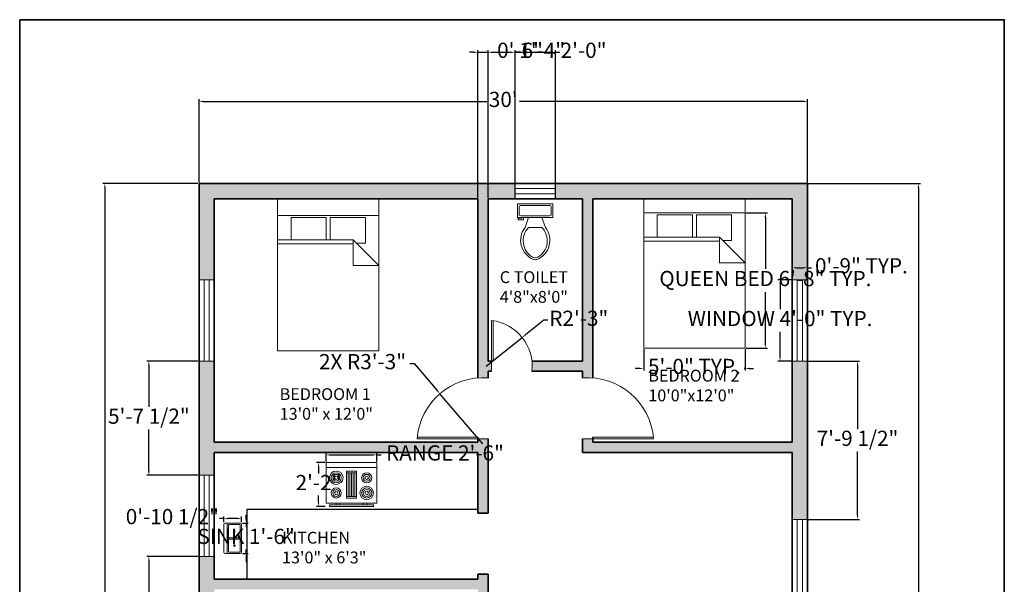
# Model space of a CAD drawing. Units: inches. Extents: x 1994 to 2577, y 1461 to 2158.
# Tile 2 of 2: x 1994 to 2577, y 1824 to 2158. Entities that reach past the tile are written whole.
import ezdxf

# ---------------------------------------------------------------- set-up
doc = ezdxf.new("R2010")
doc.units = ezdxf.units.IN
for name, color, linetype, lineweight in [('A-ANNO-DIMS', 2, 'Continuous', 18), ('A-ANNO-TTLB', 7, 'Continuous', 35), ('A-AREA-IDEN', 7, 'Continuous', 18), ('A-DOOR', 3, 'Continuous', 18), ('A-EQPM', 9, 'Continuous', 18), ('A-FLOR-CASE', 7, 'Continuous', 25), ('A-FLOR-FIXT', 9, 'Continuous', 18), ('A-FURN', 9, 'Continuous', 18), ('A-GLAZ', 4, 'Continuous', 18), ('A-WALL', 7, 'Continuous', 35), ('A-WALL-PATT', 8, 'Continuous', 13)]:
    doc.layers.add(name, color=color, linetype=linetype, lineweight=lineweight)
doc.styles.get("Standard").update_dxf_attribs({"font": 'arial.ttf'})
doc.dimstyles.new('ISO-25', dxfattribs={"dimtxt": 9, "dimasz": 2.5, "dimexe": 1.25, "dimexo": 0.625, "dimgap": 2, "dimtad": 0, "dimtih": 1, "dimtoh": 1, "dimdec": 1, "dimlunit": 4, "dimtxsty": 'Standard', "dimcen": 2.5, "dimadec": 0, "dimazin": 0, "dimtfac": 1, "dimtdec": 1, "dimtmove": 0, "dimatfit": 3, "dimfxl": 1, "dimarcsym": 0})

# ---------------------------------------------------------------- blocks, each defined once
blk = doc.blocks.new('Bed - Queen')
for p, q in [((0, -80.00003), (0, 0)), ((0, 0), (59.99999, 0)), ((59.99999, 0), (59.99999, -80.00003)), ((7.99999, -1.2), (28.79998, -1.2)), ((7.99999, -14.4), (7.99999, -1.2)), ((28.79998, -1.2), (28.79998, -14.4)), ((31.19999, -1.2), (51.99999, -1.2)), ((31.19999, -14.4), (31.19999, -1.2)), ((51.99999, -1.2), (51.99999, -16.4)), ((0, -14.4), (44.8, -14.4)), ((44.8, -16.8), (0, -16.8)), ((59.99999, -29.6), (44.8, -14.4)), ((44.8, -14.4), (44.8, -29.6)), ((51.99999, -16.4), (46.79936, -16.4)), ((44.8, -29.6), (59.99999, -29.6)), ((59.99999, -80.00003), (0, -80.00003))]:
    blk.add_line(p, q)
blk = doc.blocks.new('Sink-double - 36 in top')
for p, q in [((-18, -4), (18, -4)), ((-0.75, -18.5), (-0.75, -6.5)), ((0.75, -6.5), (0.75, -18.5))]:
    blk.add_line(p, q)
for points in [[(-16.5, 0), (16.5, 0)], [(-18, -19.5), (-18, -1.5)], [(-16.5, -18.5), (-16.5, -6.5)], [(-15.5, -5.5), (-1.75, -5.5)], [(1.75, -5.5), (15.5, -5.5)], [(16.5, -6.5), (16.5, -18.5)], [(18, -1.5), (18, -19.5)], [(16.5, -21), (-16.5, -21)], [(-1.75, -19.5), (-15.5, -19.5)], [(15.5, -19.5), (1.75, -19.5)]]:
    blk.add_lwpolyline(points)
for centre, radius in [((-8.5, -12.5), 1), ((8.5, -12.5), 1), ((-8.5, -12.5), 0.5), ((8.5, -12.5), 0.5)]:
    blk.add_circle(centre, radius)
for centre, radius, start, end in [((-16.5, -1.5), 1.5, 90, 180), ((16.5, -1.5), 1.5, 0, 90), ((-15.5, -6.5), 1, 90, 180), ((-1.75, -6.5), 1, 0, 90), ((1.75, -6.5), 1, 90, 180), ((15.5, -6.5), 1, 0, 90), ((-16.5, -19.5), 1.5, 180, 270), ((-15.5, -18.5), 1, 180, 270), ((-1.75, -18.5), 1, 270, 0), ((1.75, -18.5), 1, 180, 270), ((15.5, -18.5), 1, 270, 0), ((16.5, -19.5), 1.5, 270, 0)]:
    blk.add_arc(centre, radius, start, end)
blk = doc.blocks.new('Range-Oven - 30 in top')
for p, q in [((0, -3), (30, -3)), ((12, -6), (18, -6)), ((13, -20), (13, -6)), ((14, -6), (14, -20)), ((15, -20), (15, -6)), ((16, -6), (16, -20)), ((17, -20), (17, -6)), ((18, -20), (12, -20)), ((6, -24), (6, -25)), ((8, -25), (8, -24)), ((22, -25), (22, -24)), ((24, -24), (24, -25))]:
    blk.add_line(p, q)
for points in [[(0, -24), (0, 0), (30, 0), (30, -24)], [(12, -21), (12, -5), (18, -5), (18, -21)], [(2, -26), (2, -25), (28, -25), (28, -26)]]:
    blk.add_lwpolyline(points, close=True)
for centre, radius in [((6, -9), 4), ((6, -9), 3), ((6, -9), 2), ((6, -9), 1), ((24, -9), 3), ((24, -9), 2), ((24, -9), 1), ((6, -18), 3), ((6, -18), 2), ((6, -18), 1), ((24, -18), 4), ((24, -18), 3), ((24, -18), 2), ((24, -18), 1)]:
    blk.add_circle(centre, radius)
blk = doc.blocks.new('*D4')
at = {"layer": 'A-ANNO-DIMS', "color": 0, "lineweight": -2, "transparency": 16777216}
for p, q in [((2461.02, 2061.02), (2527.29, 2061.02)), ((2526.04, 2058.52), (2526.04, 1797.59)), ((2526.04, 1523.52), (2526.04, 1784.44)), ((2461.02, 1521.02), (2527.29, 1521.02))]:
    blk.add_line(p, q, dxfattribs=at)
at = {"layer": 'A-ANNO-DIMS', "color": 0, "transparency": 16777216}
for points in [[(2525.63, 2058.52), (2526.46, 2058.52), (2526.04, 2061.02)], [(2525.63, 1523.52), (2526.46, 1523.52), (2526.04, 1521.02)]]:
    blk.add_solid(points, dxfattribs=at)
at = {"layer": 'Defpoints', "color": 0, "transparency": 16777216}
for p in [(2460.39, 2061.02), (2460.39, 1521.02), (2526.04, 1521.02)]:
    blk.add_point(p, dxfattribs=at)
at = {"layer": 'A-ANNO-DIMS', "color": 0, "transparency": 16777216, "insert": (2526.04, 1791.02), "char_height": 9, "attachment_point": 5}
blk.add_mtext("45'", dxfattribs=at)
blk = doc.blocks.new('*D5')
at = {"layer": 'A-ANNO-DIMS', "color": 0, "lineweight": -2, "transparency": 16777216}
for p, q in [((2100.39, 2061.64), (2100.39, 2110.85)), ((2102.89, 2109.6), (2270.76, 2109.6)), ((2457.89, 2109.6), (2290.02, 2109.6)), ((2460.39, 2061.64), (2460.39, 2110.85))]:
    blk.add_line(p, q, dxfattribs=at)
at = {"layer": 'A-ANNO-DIMS', "color": 0, "transparency": 16777216}
for points in [[(2102.89, 2110.02), (2102.89, 2109.18), (2100.39, 2109.6)], [(2457.89, 2110.02), (2457.89, 2109.18), (2460.39, 2109.6)]]:
    blk.add_solid(points, dxfattribs=at)
at = {"layer": 'Defpoints', "color": 0, "transparency": 16777216}
for p in [(2460.39, 2109.6), (2100.39, 2061.02), (2460.39, 2061.02)]:
    blk.add_point(p, dxfattribs=at)
at = {"layer": 'A-ANNO-DIMS', "color": 0, "transparency": 16777216, "insert": (2280.39, 2109.6), "char_height": 9, "attachment_point": 5}
blk.add_mtext("30'", dxfattribs=at)
blk = doc.blocks.new('*U7')
for p, q in [((9.5, -6), (9.5, -2)), ((-10, -8.5), (-8, -8.5)), ((-10, -9.5), (-10, -8.5)), ((-7, -9.5), (-10, -9.5)), ((-8, -8.5), (-8, -8)), ((-7, -8), (-7, -9.5)), ((-4, -8), (-6, -14)), ((4, -8), (6, -14)), ((4, -14), (-4, -14))]:
    blk.add_line(p, q)
blk.add_lwpolyline([(10.5, -8), (10.5, 0), (-10.5, 0), (-10.5, -8)], close=True)
for points in [[(-9.5, -2), (-9.5, -6)], [(8.5, -1), (-8.5, -1)], [(-8.5, -7), (8.5, -7)]]:
    blk.add_lwpolyline(points)
for centre, radius, start, end in [((-8.62, -1.88), 0.884, 81.8699, 188.1301), ((8.62, -1.88), 0.884, 351.8699, 98.1301), ((-8.62, -6.12), 0.884, 171.8699, 278.1301), ((8.62, -6.12), 0.884, 261.8699, 8.1301), ((3.52, -21.58), 12.17, 141.46911, 247.97143), ((4.2, -21.82), 11.33, 136.36773, 238.94682), ((-3.52, -21.58), 12.17, 292.02843, 38.53071), ((-4.2, -21.82), 11.33, 301.05301, 43.63209), ((0, -27.88), 4, 245.73182, 294.26817), ((0, -29), 4, 254.86053, 285.13947)]:
    blk.add_arc(centre, radius, start, end)
blk = doc.blocks.new('*D8')
at = {"layer": 'A-ANNO-DIMS', "color": 0, "lineweight": -2, "transparency": 16777216}
for p, q in [((2099.77, 2061.02), (2043.44, 2061.02)), ((2044.69, 2058.52), (2044.69, 1797.59)), ((2044.69, 1523.52), (2044.69, 1784.44)), ((2099.77, 1521.02), (2043.44, 1521.02))]:
    blk.add_line(p, q, dxfattribs=at)
at = {"layer": 'A-ANNO-DIMS', "color": 0, "transparency": 16777216}
for points in [[(2044.27, 2058.52), (2045.11, 2058.52), (2044.69, 2061.02)], [(2044.27, 1523.52), (2045.11, 1523.52), (2044.69, 1521.02)]]:
    blk.add_solid(points, dxfattribs=at)
at = {"layer": 'Defpoints', "color": 0, "transparency": 16777216}
for p in [(2100.39, 2061.02), (2044.69, 1521.02), (2100.39, 1521.02)]:
    blk.add_point(p, dxfattribs=at)
at = {"layer": 'A-ANNO-DIMS', "color": 0, "transparency": 16777216, "insert": (2044.69, 1791.02), "char_height": 9, "attachment_point": 5}
blk.add_mtext("45'", dxfattribs=at)
blk = doc.blocks.new('WIN-48IN')
for p, q in [((9, 48), (0, 48)), ((0, 48), (0, 0)), ((3, 48), (3, 0)), ((6, 48), (6, 0)), ((9, 0), (0, 0))]:
    blk.add_line(p, q)
blk = doc.blocks.new('DOOR-SWING-36IN')
for p, q in [((36, 1), (0, 1)), ((36, 0), (0, 0)), ((36, 0), (42, 0))]:
    blk.add_line(p, q)
blk.add_arc((39, -3), 39.12, 85.60129, 175.60129)
blk = doc.blocks.new('*D11')
at = {"layer": 'A-ANNO-DIMS', "color": 0, "lineweight": -2, "transparency": 16777216}
for p, q in [((2450.77, 2004.02), (2442.94, 2004.02)), ((2444.19, 2001.52), (2444.19, 1986.67)), ((2444.19, 1958.52), (2444.19, 1973.36)), ((2450.77, 1956.02), (2442.94, 1956.02))]:
    blk.add_line(p, q, dxfattribs=at)
at = {"layer": 'A-ANNO-DIMS', "color": 0, "transparency": 16777216}
for points in [[(2443.77, 2001.52), (2444.61, 2001.52), (2444.19, 2004.02)], [(2443.77, 1958.52), (2444.61, 1958.52), (2444.19, 1956.02)]]:
    blk.add_solid(points, dxfattribs=at)
at = {"layer": 'Defpoints', "color": 0, "transparency": 16777216}
for p in [(2444.19, 2004.02), (2451.39, 2004.02), (2451.39, 1956.02)]:
    blk.add_point(p, dxfattribs=at)
at = {"layer": 'A-ANNO-DIMS', "color": 0, "transparency": 16777216, "insert": (2444.19, 1980.02), "char_height": 9, "attachment_point": 5}
blk.add_mtext('WINDOW 4\'-0" TYP.', dxfattribs=at)
blk = doc.blocks.new('*D12')
at = {"layer": 'A-ANNO-DIMS', "color": 0, "lineweight": -2, "transparency": 16777216}
for p, q in [((2451.39, 2004.64), (2451.39, 2012.47)), ((2453.89, 2011.22), (2457.89, 2011.22)), ((2460.39, 2004.64), (2460.39, 2012.47)), ((2460.39, 2011.22), (2462.89, 2011.22))]:
    blk.add_line(p, q, dxfattribs=at)
at = {"layer": 'A-ANNO-DIMS', "color": 0, "transparency": 16777216}
for points in [[(2453.89, 2011.63), (2453.89, 2010.8), (2451.39, 2011.22)], [(2457.89, 2011.63), (2457.89, 2010.8), (2460.39, 2011.22)]]:
    blk.add_solid(points, dxfattribs=at)
at = {"layer": 'Defpoints', "color": 0, "transparency": 16777216}
for p in [(2460.39, 2011.22), (2451.39, 2004.02), (2460.39, 2004.02)]:
    blk.add_point(p, dxfattribs=at)
at = {"layer": 'A-ANNO-DIMS', "color": 0, "transparency": 16777216, "insert": (2492.32, 2011.22), "char_height": 9, "attachment_point": 5}
blk.add_mtext('0\'-9" TYP.', dxfattribs=at)
blk = doc.blocks.new('*D15')
at = {"layer": 'A-ANNO-DIMS', "color": 0, "lineweight": -2, "transparency": 16777216}
for p, q in [((2424.13, 2043.69), (2436.75, 2043.69)), ((2435.5, 2041.19), (2435.5, 2010.62)), ((2435.5, 1966.19), (2435.5, 1996.76)), ((2424.13, 1963.69), (2436.75, 1963.69))]:
    blk.add_line(p, q, dxfattribs=at)
at = {"layer": 'A-ANNO-DIMS', "color": 0, "transparency": 16777216}
for points in [[(2435.09, 2041.19), (2435.92, 2041.19), (2435.5, 2043.69)], [(2435.09, 1966.19), (2435.92, 1966.19), (2435.5, 1963.69)]]:
    blk.add_solid(points, dxfattribs=at)
at = {"layer": 'Defpoints', "color": 0, "transparency": 16777216}
for p in [(2423.5, 2043.69), (2435.5, 2043.69), (2423.5, 1963.69)]:
    blk.add_point(p, dxfattribs=at)
at = {"layer": 'A-ANNO-DIMS', "color": 0, "transparency": 16777216, "insert": (2435.5, 2003.69), "char_height": 9, "attachment_point": 5}
blk.add_mtext('QUEEN BED 6\'-8" TYP.', dxfattribs=at)
blk = doc.blocks.new('*D16')
at = {"layer": 'A-ANNO-DIMS', "color": 0, "lineweight": -2, "transparency": 16777216}
for p, q in [((2363.5, 1963.07), (2363.5, 1950.44)), ((2423.5, 1963.07), (2423.5, 1950.44)), ((2361, 1951.69), (2358.5, 1951.69)), ((2363.5, 1951.69), (2364.07, 1951.69)), ((2423.5, 1951.69), (2422.93, 1951.69)), ((2426, 1951.69), (2428.5, 1951.69))]:
    blk.add_line(p, q, dxfattribs=at)
at = {"layer": 'A-ANNO-DIMS', "color": 0, "transparency": 16777216}
for points in [[(2361, 1952.11), (2361, 1951.28), (2363.5, 1951.69)], [(2426, 1952.11), (2426, 1951.28), (2423.5, 1951.69)]]:
    blk.add_solid(points, dxfattribs=at)
at = {"layer": 'Defpoints', "color": 0, "transparency": 16777216}
for p in [(2363.5, 1963.69), (2423.5, 1963.69), (2423.5, 1951.69)]:
    blk.add_point(p, dxfattribs=at)
at = {"layer": 'A-ANNO-DIMS', "color": 0, "transparency": 16777216, "insert": (2393.5, 1951.69), "char_height": 9, "attachment_point": 5}
blk.add_mtext('5\'-0" TYP.', dxfattribs=at)
blk = doc.blocks.new('*D17')
at = {"layer": 'A-ANNO-DIMS', "color": 0, "lineweight": -2, "transparency": 16777216}
for p, q in [((2128.26, 1862.68), (2128.26, 1865.18)), ((2126.19, 1860.18), (2129.51, 1860.18)), ((2128.26, 1860.18), (2128.26, 1857.84)), ((2126.19, 1842.18), (2129.51, 1842.18)), ((2128.26, 1842.18), (2128.26, 1844.53)), ((2128.26, 1839.68), (2128.26, 1837.18))]:
    blk.add_line(p, q, dxfattribs=at)
at = {"layer": 'A-ANNO-DIMS', "color": 0, "transparency": 16777216}
for points in [[(2127.85, 1862.68), (2128.68, 1862.68), (2128.26, 1860.18)], [(2127.85, 1839.68), (2128.68, 1839.68), (2128.26, 1842.18)]]:
    blk.add_solid(points, dxfattribs=at)
at = {"layer": 'Defpoints', "color": 0, "transparency": 16777216}
for p in [(2125.57, 1860.18), (2128.26, 1860.18), (2125.57, 1842.18)]:
    blk.add_point(p, dxfattribs=at)
at = {"layer": 'A-ANNO-DIMS', "color": 0, "transparency": 16777216, "insert": (2128.26, 1851.18), "char_height": 9, "attachment_point": 5}
blk.add_mtext('SINK 1\'-6"', dxfattribs=at)
blk = doc.blocks.new('*D18')
at = {"layer": 'A-ANNO-DIMS', "color": 0, "lineweight": -2, "transparency": 16777216}
for p, q in [((2115.07, 1862.88), (2112.57, 1862.88)), ((2115.07, 1860.81), (2115.07, 1864.13)), ((2123.07, 1862.88), (2117.57, 1862.88)), ((2125.57, 1860.81), (2125.57, 1864.13))]:
    blk.add_line(p, q, dxfattribs=at)
at = {"layer": 'A-ANNO-DIMS', "color": 0, "transparency": 16777216}
for points in [[(2117.57, 1863.3), (2117.57, 1862.46), (2115.07, 1862.88)], [(2123.07, 1863.3), (2123.07, 1862.46), (2125.57, 1862.88)]]:
    blk.add_solid(points, dxfattribs=at)
at = {"layer": 'Defpoints', "color": 0, "transparency": 16777216}
for p in [(2115.07, 1862.88), (2115.07, 1860.18), (2125.57, 1860.18)]:
    blk.add_point(p, dxfattribs=at)
at = {"layer": 'A-ANNO-DIMS', "color": 0, "transparency": 16777216, "insert": (2084.62, 1862.88), "char_height": 9, "attachment_point": 5}
blk.add_mtext('0\'-10 1/2"', dxfattribs=at)
blk = doc.blocks.new('*D19')
at = {"layer": 'A-ANNO-DIMS', "color": 0, "lineweight": -2, "transparency": 16777216}
for p, q in [((2175.6, 1896.64), (2175.6, 1901.77)), ((2178.1, 1900.52), (2203.1, 1900.52)), ((2205.6, 1896.64), (2205.6, 1901.77)), ((2205.6, 1900.52), (2208.1, 1900.52))]:
    blk.add_line(p, q, dxfattribs=at)
at = {"layer": 'A-ANNO-DIMS', "color": 0, "transparency": 16777216}
for points in [[(2178.1, 1900.94), (2178.1, 1900.1), (2175.6, 1900.52)], [(2203.1, 1900.94), (2203.1, 1900.1), (2205.6, 1900.52)]]:
    blk.add_solid(points, dxfattribs=at)
at = {"layer": 'Defpoints', "color": 0, "transparency": 16777216}
for p in [(2205.6, 1900.52), (2175.6, 1896.02), (2205.6, 1896.02)]:
    blk.add_point(p, dxfattribs=at)
at = {"layer": 'A-ANNO-DIMS', "color": 0, "transparency": 16777216, "insert": (2245.93, 1900.52), "char_height": 9, "attachment_point": 5}
blk.add_mtext('RANGE 2\'-6"', dxfattribs=at)
blk = doc.blocks.new('*D20')
at = {"layer": 'A-ANNO-DIMS', "color": 0, "lineweight": -2, "transparency": 16777216}
for p, q in [((2174.98, 1896.02), (2169.85, 1896.02)), ((2171.1, 1893.52), (2171.1, 1889.54)), ((2171.1, 1872.52), (2171.1, 1876.5)), ((2174.98, 1870.02), (2169.85, 1870.02))]:
    blk.add_line(p, q, dxfattribs=at)
at = {"layer": 'A-ANNO-DIMS', "color": 0, "transparency": 16777216}
for points in [[(2170.69, 1893.52), (2171.52, 1893.52), (2171.1, 1896.02)], [(2170.69, 1872.52), (2171.52, 1872.52), (2171.1, 1870.02)]]:
    blk.add_solid(points, dxfattribs=at)
at = {"layer": 'Defpoints', "color": 0, "transparency": 16777216}
for p in [(2171.1, 1896.02), (2175.6, 1896.02), (2175.6, 1870.02)]:
    blk.add_point(p, dxfattribs=at)
at = {"layer": 'A-ANNO-DIMS', "color": 0, "transparency": 16777216, "insert": (2171.1, 1883.02), "char_height": 9, "attachment_point": 5}
blk.add_mtext('2\'-2"', dxfattribs=at)
blk = doc.blocks.new('*D22')
at = {"layer": 'A-ANNO-DIMS', "color": 0, "lineweight": -2, "transparency": 16777216}
for p, q in [((2262.89, 2138.65), (2260.39, 2138.65)), ((2265.39, 2052.64), (2265.39, 2139.9)), ((2265.39, 2138.65), (2271.39, 2138.65)), ((2271.39, 2052.64), (2271.39, 2139.9)), ((2273.89, 2138.65), (2276.39, 2138.65))]:
    blk.add_line(p, q, dxfattribs=at)
at = {"layer": 'A-ANNO-DIMS', "color": 0, "transparency": 16777216}
for points in [[(2262.89, 2139.07), (2262.89, 2138.23), (2265.39, 2138.65)], [(2273.89, 2139.07), (2273.89, 2138.23), (2271.39, 2138.65)]]:
    blk.add_solid(points, dxfattribs=at)
at = {"layer": 'Defpoints', "color": 0, "transparency": 16777216}
for p in [(2271.39, 2138.65), (2265.39, 2052.02), (2271.39, 2052.02)]:
    blk.add_point(p, dxfattribs=at)
at = {"layer": 'A-ANNO-DIMS', "color": 0, "transparency": 16777216, "insert": (2290.35, 2138.65), "char_height": 9, "attachment_point": 5}
blk.add_mtext('0\'-6"', dxfattribs=at)
blk = doc.blocks.new('*D29')
at = {"layer": 'A-ANNO-DIMS', "color": 0, "lineweight": -2, "transparency": 16777216}
for p, q in [((2461.02, 1956.02), (2491.29, 1956.02)), ((2490.04, 1953.52), (2490.04, 1915.83)), ((2490.04, 1864.84), (2490.04, 1902.53)), ((2461.02, 1862.34), (2491.29, 1862.34))]:
    blk.add_line(p, q, dxfattribs=at)
at = {"layer": 'A-ANNO-DIMS', "color": 0, "transparency": 16777216}
for points in [[(2489.62, 1953.52), (2490.46, 1953.52), (2490.04, 1956.02)], [(2489.62, 1864.84), (2490.46, 1864.84), (2490.04, 1862.34)]]:
    blk.add_solid(points, dxfattribs=at)
at = {"layer": 'Defpoints', "color": 0, "transparency": 16777216}
for p in [(2460.39, 1956.02), (2490.04, 1956.02), (2460.39, 1862.34)]:
    blk.add_point(p, dxfattribs=at)
at = {"layer": 'A-ANNO-DIMS', "color": 0, "transparency": 16777216, "insert": (2490.04, 1909.18), "char_height": 9, "attachment_point": 5}
blk.add_mtext('7\'-9 1/2"', dxfattribs=at)
blk = doc.blocks.new('*D31')
at = {"layer": 'A-ANNO-DIMS', "color": 0, "lineweight": -2, "transparency": 16777216}
for p, q in [((2099.77, 1840.52), (2069.49, 1840.52)), ((2070.74, 1838.02), (2070.74, 1816.42)), ((2070.74, 1781.52), (2070.74, 1803.11)), ((2099.77, 1779.02), (2069.49, 1779.02))]:
    blk.add_line(p, q, dxfattribs=at)
at = {"layer": 'A-ANNO-DIMS', "color": 0, "transparency": 16777216}
for points in [[(2070.32, 1838.02), (2071.16, 1838.02), (2070.74, 1840.52)], [(2070.32, 1781.52), (2071.16, 1781.52), (2070.74, 1779.02)]]:
    blk.add_solid(points, dxfattribs=at)
at = {"layer": 'Defpoints', "color": 0, "transparency": 16777216}
for p in [(2070.74, 1840.52), (2100.39, 1840.52), (2100.39, 1779.02)]:
    blk.add_point(p, dxfattribs=at)
at = {"layer": 'A-ANNO-DIMS', "color": 0, "transparency": 16777216, "insert": (2070.74, 1809.77), "char_height": 9, "attachment_point": 5}
blk.add_mtext('5\'-1 1/2"', dxfattribs=at)
blk = doc.blocks.new('*D32')
at = {"layer": 'A-ANNO-DIMS', "color": 0, "lineweight": -2, "transparency": 16777216}
for p, q in [((2099.77, 1956.02), (2069.49, 1956.02)), ((2070.74, 1953.52), (2070.74, 1928.92)), ((2070.74, 1891.02), (2070.74, 1915.61)), ((2099.77, 1888.52), (2069.49, 1888.52))]:
    blk.add_line(p, q, dxfattribs=at)
at = {"layer": 'A-ANNO-DIMS', "color": 0, "transparency": 16777216}
for points in [[(2070.32, 1953.52), (2071.16, 1953.52), (2070.74, 1956.02)], [(2070.32, 1891.02), (2071.16, 1891.02), (2070.74, 1888.52)]]:
    blk.add_solid(points, dxfattribs=at)
at = {"layer": 'Defpoints', "color": 0, "transparency": 16777216}
for p in [(2070.74, 1956.02), (2100.39, 1956.02), (2100.39, 1888.52)]:
    blk.add_point(p, dxfattribs=at)
at = {"layer": 'A-ANNO-DIMS', "color": 0, "transparency": 16777216, "insert": (2070.74, 1922.27), "char_height": 9, "attachment_point": 5}
blk.add_mtext('5\'-7 1/2"', dxfattribs=at)
blk = doc.blocks.new('*D33')
at = {"layer": 'A-ANNO-DIMS', "color": 0, "lineweight": -2, "transparency": 16777216}
for p, q in [((2287.39, 2052.64), (2287.39, 2139.9)), ((2289.89, 2138.65), (2308.89, 2138.65)), ((2311.39, 2052.64), (2311.39, 2139.9)), ((2311.39, 2138.65), (2313.89, 2138.65))]:
    blk.add_line(p, q, dxfattribs=at)
at = {"layer": 'A-ANNO-DIMS', "color": 0, "transparency": 16777216}
for points in [[(2289.89, 2139.07), (2289.89, 2138.23), (2287.39, 2138.65)], [(2308.89, 2139.07), (2308.89, 2138.23), (2311.39, 2138.65)]]:
    blk.add_solid(points, dxfattribs=at)
at = {"layer": 'Defpoints', "color": 0, "transparency": 16777216}
for p in [(2311.39, 2138.65), (2287.39, 2052.02), (2311.39, 2052.02)]:
    blk.add_point(p, dxfattribs=at)
at = {"layer": 'A-ANNO-DIMS', "color": 0, "transparency": 16777216, "insert": (2327.93, 2138.65), "char_height": 9, "attachment_point": 5}
blk.add_mtext('2\'-0"', dxfattribs=at)
blk = doc.blocks.new('*D34')
at = {"layer": 'A-ANNO-DIMS', "color": 0, "lineweight": -2, "transparency": 16777216}
for p, q in [((2271.39, 2052.64), (2271.39, 2139.9)), ((2273.89, 2138.65), (2284.89, 2138.65)), ((2287.39, 2052.64), (2287.39, 2139.9)), ((2287.39, 2138.65), (2289.89, 2138.65))]:
    blk.add_line(p, q, dxfattribs=at)
at = {"layer": 'A-ANNO-DIMS', "color": 0, "transparency": 16777216}
for points in [[(2273.89, 2139.07), (2273.89, 2138.23), (2271.39, 2138.65)], [(2284.89, 2139.07), (2284.89, 2138.23), (2287.39, 2138.65)]]:
    blk.add_solid(points, dxfattribs=at)
at = {"layer": 'Defpoints', "color": 0, "transparency": 16777216}
for p in [(2287.39, 2138.65), (2271.39, 2052.02), (2287.39, 2052.02)]:
    blk.add_point(p, dxfattribs=at)
at = {"layer": 'A-ANNO-DIMS', "color": 0, "transparency": 16777216, "insert": (2303.43, 2138.65), "char_height": 9, "attachment_point": 5}
blk.add_mtext('1\'-4"', dxfattribs=at)
blk = doc.blocks.new('*D40')
at = {"layer": 'A-ANNO-DIMS', "color": 0, "lineweight": -2, "transparency": 16777216}
for p, q in [((2225.16, 1954.53), (2227.66, 1954.53)), ((2227.66, 1954.53), (2241.31, 1938.61)), ((2268.39, 1907.02), (2242.93, 1936.71))]:
    blk.add_line(p, q, dxfattribs=at)
at = {"layer": 'A-ANNO-DIMS', "color": 0, "transparency": 16777216}
blk.add_solid([(2241.62, 1938.88), (2240.99, 1938.34), (2242.93, 1936.71)], dxfattribs=at)
at = {"layer": 'Defpoints', "color": 0, "transparency": 16777216}
for p in [(2242.93, 1936.71), (2268.39, 1907.02)]:
    blk.add_point(p, dxfattribs=at)
at = {"layer": 'A-ANNO-DIMS', "color": 0, "transparency": 16777216, "insert": (2197.15, 1954.53), "char_height": 9, "attachment_point": 5}
blk.add_mtext('2X R3\'-3"', dxfattribs=at)
blk = doc.blocks.new('*D41')
at = {"layer": 'A-ANNO-DIMS', "color": 0, "lineweight": -2, "transparency": 16777216}
for p, q in [((2304.33, 1980.17), (2293.56, 1971.55)), ((2306.83, 1980.17), (2304.33, 1980.17)), ((2270.39, 1953.02), (2291.6, 1969.99))]:
    blk.add_line(p, q, dxfattribs=at)
at = {"layer": 'A-ANNO-DIMS', "color": 0, "transparency": 16777216}
blk.add_solid([(2293.3, 1971.87), (2293.82, 1971.22), (2291.6, 1969.99)], dxfattribs=at)
at = {"layer": 'Defpoints', "color": 0, "transparency": 16777216}
for p in [(2291.6, 1969.99), (2270.39, 1953.02)]:
    blk.add_point(p, dxfattribs=at)
at = {"layer": 'A-ANNO-DIMS', "color": 0, "transparency": 16777216, "insert": (2325.1, 1980.17), "char_height": 9, "attachment_point": 5}
blk.add_mtext('R2\'-3"', dxfattribs=at)

msp = doc.modelspace()

# ---------------------------------------------------------------- hatches: boundary and pattern name
at = {"layer": 'A-WALL-PATT'}
h = msp.add_hatch(color=256, dxfattribs=at)
h.dxf.hatch_style = 1
h.paths.add_polyline_path([(2287.39, 2061.02), (2100.39, 2061.02), (2100.39, 2004.02), (2109.39, 2004.02), (2109.39, 2052.02), (2265.39, 2052.02), (2265.39, 1946.02, -0.038405), (2271.39, 1946.02), (2271.39, 1950.02), (2273.39, 1950.02), (2273.39, 1956.02), (2271.39, 1956.02), (2271.39, 2052.02), (2287.39, 2052.02)])
h.paths.add_polyline_path([(2460.39, 2061.02), (2311.39, 2061.02), (2311.39, 2052.02), (2327.39, 2052.02), (2327.39, 1956.02), (2297.39, 1956.02, -0.055385), (2297.39, 1950.02), (2327.39, 1950.02), (2327.39, 1946.02, -0.038405), (2333.39, 1946.02), (2333.39, 2052.02), (2451.39, 2052.02), (2451.39, 2004.02), (2460.39, 2004.02)])
h.paths.add_polyline_path([(2460.39, 1956.02), (2451.39, 1956.02), (2451.39, 1908.02), (2333.39, 1908.02), (2333.39, 1910.02), (2327.39, 1910.02), (2327.39, 1902.02), (2451.39, 1902.02), (2451.39, 1862.34), (2460.39, 1862.34)])
h.paths.add_polyline_path([(2109.39, 1956.02), (2100.39, 1956.02), (2100.39, 1888.52), (2109.39, 1888.52), (2109.39, 1902.02), (2265.39, 1902.02), (2265.39, 1866.02), (2271.39, 1866.02), (2271.39, 1910.02), (2265.39, 1910.02), (2265.39, 1908.02), (2109.39, 1908.02)])
h.paths.add_polyline_path([(2460.39, 1814.34), (2451.39, 1814.34), (2451.39, 1686.53), (2460.39, 1686.53)])
h.paths.add_polyline_path([(2271.39, 1830.02), (2265.39, 1830.02), (2265.39, 1827.02), (2109.39, 1827.02), (2109.39, 1840.52), (2100.39, 1840.52), (2100.39, 1779.02), (2109.39, 1779.02), (2109.39, 1821.02), (2265.39, 1821.02), (2265.39, 1729.02, -0.038405), (2271.39, 1729.02)])
h.paths.add_polyline_path([(2109.39, 1683.02), (2265.39, 1683.02), (2265.39, 1679.02), (2271.39, 1679.02), (2271.39, 1693.02), (2265.39, 1693.02), (2265.39, 1689.02), (2109.39, 1689.02), (2109.39, 1731.02), (2100.39, 1731.02), (2100.39, 1521.02), (2163.39, 1521.02), (2163.39, 1530.02), (2109.39, 1530.02)])
h.paths.add_polyline_path([(2273.39, 1530.02), (2271.39, 1530.02), (2271.39, 1606.02), (2273.39, 1606.02, -0.038405), (2273.39, 1612.02), (2271.39, 1612.02), (2271.39, 1643.02, -0.038405), (2265.39, 1643.02), (2265.39, 1530.02), (2211.39, 1530.02), (2211.39, 1521.02), (2273.39, 1521.02)])
h.paths.add_polyline_path([(2460.39, 1544.02), (2451.39, 1544.02), (2451.39, 1530.02), (2309.39, 1530.02, -0.055385), (2309.39, 1521.02), (2460.39, 1521.02)])
h.paths.add_polyline_path([(2460.39, 1638.53), (2451.39, 1638.53), (2451.39, 1612.02), (2309.39, 1612.02), (2309.39, 1606.02), (2451.39, 1606.02), (2451.39, 1592.02), (2460.39, 1592.02)])

# ---------------------------------------------------------------- linework, layer by layer
at = {"layer": 'A-ANNO-TTLB'}
msp.add_lwpolyline([(1994.29, 2157.92), (2576.88, 2157.92), (2576.88, 1461.09), (1994.29, 1461.09)], close=True, dxfattribs=at)
at = {"layer": 'A-DOOR'}
for p, q in [((2273.39, 1956.02), (2273.39, 1980.02)), ((2274.39, 1956.02), (2274.39, 1980.02)), ((2273.39, 1956.02), (2273.39, 1950.02))]:
    msp.add_line(p, q, dxfattribs=at)
msp.add_arc((2270.39, 1953.02), 27.17, 353.65981, 83.65981, dxfattribs=at)
at = {"layer": 'A-FLOR-CASE'}
for p, q in [((2265.39, 1868.28), (2128.61, 1868.28)), ((2128.61, 1868.28), (2128.61, 1827.02))]:
    msp.add_line(p, q, dxfattribs=at)
at = {"layer": 'A-FURN'}
for p, q in [((2146.85, 2042.17), (2146.85, 2052.02)), ((2206.85, 2042.17), (2206.85, 2052.02)), ((2363.5, 2043.69), (2363.5, 2052.02)), ((2423.5, 2043.69), (2423.5, 2052.02))]:
    msp.add_line(p, q, dxfattribs=at)
at = {"layer": 'A-GLAZ'}
for p, q in [((2287.39, 2052.02), (2287.39, 2061.02)), ((2287.39, 2058.02), (2311.39, 2058.02)), ((2311.39, 2052.02), (2311.39, 2061.02)), ((2287.39, 2055.02), (2311.39, 2055.02)), ((2287.39, 2052.02), (2311.39, 2052.02)), ((2287.39, 2052.02), (2311.39, 2052.02))]:
    msp.add_line(p, q, dxfattribs=at)
at = {"layer": 'A-WALL'}
for p, q in [((2100.39, 2061.02), (2460.39, 2061.02)), ((2100.39, 1521.02), (2100.39, 2061.02)), ((2460.39, 2061.02), (2460.39, 1521.02)), ((2109.39, 2052.02), (2265.39, 2052.02)), ((2109.39, 1908.02), (2109.39, 2052.02)), ((2265.39, 1946.02), (2265.39, 2052.02)), ((2271.39, 1956.02), (2271.39, 2052.02)), ((2271.39, 2052.02), (2327.39, 2052.02)), ((2327.39, 1956.02), (2327.39, 2052.02)), ((2333.39, 2052.02), (2451.39, 2052.02)), ((2333.39, 1946.02), (2333.39, 2052.02)), ((2333.39, 2052.02), (2451.39, 2052.02)), ((2451.39, 2052.02), (2451.39, 1908.02)), ((2271.39, 1956.02), (2274.39, 1956.02)), ((2297.39, 1956.02), (2327.39, 1956.02)), ((2271.39, 1950.02), (2273.39, 1950.02)), ((2271.39, 1946.02), (2271.39, 1950.02)), ((2297.39, 1950.02), (2327.39, 1950.02)), ((2327.39, 1946.02), (2327.39, 1950.02)), ((2265.39, 1908.02), (2265.39, 1911.02)), ((2333.39, 1908.02), (2333.39, 1911.02)), ((2109.39, 1908.02), (2265.39, 1908.02)), ((2271.39, 1866.02), (2271.39, 1910.02)), ((2327.39, 1902.02), (2327.39, 1910.02)), ((2333.39, 1908.02), (2451.39, 1908.02)), ((2109.39, 1902.02), (2265.39, 1902.02)), ((2109.39, 1827.02), (2109.39, 1902.02)), ((2265.39, 1866.02), (2265.39, 1902.02)), ((2333.39, 1902.02), (2327.39, 1902.02)), ((2451.39, 1902.02), (2327.39, 1902.02)), ((2333.39, 1902.02), (2451.39, 1902.02)), ((2451.39, 1902.02), (2451.39, 1612.02)), ((2265.39, 1866.02), (2271.39, 1866.02)), ((2265.39, 1827.02), (2265.39, 1830.02)), ((2265.39, 1830.02), (2271.39, 1830.02)), ((2271.39, 1729.02), (2271.39, 1830.02)), ((2109.39, 1827.02), (2265.39, 1827.02))]:
    msp.add_line(p, q, dxfattribs=at)

# ---------------------------------------------------------------- block references
at = {"layer": 'A-DOOR'}
msp.add_blockref('DOOR-SWING-36IN', (2229.39, 1910.02), dxfattribs=at)
at = {"layer": 'A-DOOR', "extrusion": (0, 0, -1), "zscale": -1}
msp.add_blockref('DOOR-SWING-36IN', (-2369.39, 1910.02), dxfattribs=at)
at = {"layer": 'A-EQPM'}
msp.add_blockref('Range-Oven - 30 in top', (2175.6, 1896.02), dxfattribs=at)
at = {"layer": 'A-FLOR-FIXT'}
msp.add_blockref('*U7', (2299.32, 2049), dxfattribs=at)
at = {"layer": 'A-FLOR-FIXT', "xscale": 0.4999105559057161, "yscale": 0.4999105559057161, "zscale": 0.4999105559057161, "rotation": 90}
msp.add_blockref('Sink-double - 36 in top', (2115.07, 1851.18), dxfattribs=at)
at = {"layer": 'A-FURN'}
for p in [(2146.85, 2042.17), (2363.5, 2043.69)]:
    msp.add_blockref('Bed - Queen', p, dxfattribs=at)
at = {"layer": 'A-GLAZ'}
for p in [(2100.39, 1956.02), (2451.39, 1956.02), (2100.39, 1840.52), (2451.39, 1814.34)]:
    msp.add_blockref('WIN-48IN', p, dxfattribs=at)

# ---------------------------------------------------------------- texts
at = {"layer": 'A-AREA-IDEN', "char_height": 7, "attachment_point": 1}
for s, width, insert in [('{\\fArial|b1|i0|c0|p34;C TOILET\\P4\'8"x8\'0"}', 49.0478, (2278.34, 2009.16)), ('{\\fArial|b1|i0|c0|p34;BEDROOM 2\\P10\'0"x12\'0"}', 85.1435, (2366.25, 1950.89)), ('{\\fArial|b1|i0|c0|p34;BEDROOM 1\\P13\'0" x 12\'0"}', 104.4993, (2148.13, 1939.99)), ('{\\fArial|b1|i0|c0|p34;KITCHEN\\P\\pxql;13\'0" x 6\'3"}', 99.803, (2149.53, 1855.06))]:
    msp.add_mtext_dynamic_manual_height_columns(s, width=width, gutter_width=12.5, heights=[0], dxfattribs=dict(at, insert=insert))

# ---------------------------------------------------------------- dimensions: what is measured, and where the dimension line sits
at = {"layer": 'A-ANNO-DIMS'}
for base, p1, p2, override, picture, middle in [((2271.39, 2138.65), (2265.39, 2052.02), (2271.39, 2052.02), {"dimdec": 1, "dimlfac": 1, "dimrnd": 0, "dimzin": 1, "dimdsep": 46, "dimlunit": 4, "dimfrac": 2}, '*D22', (2290.35, 2138.65)), ((2287.39, 2138.65), (2271.39, 2052.02), (2287.39, 2052.02), {"dimdec": 1, "dimlfac": 1, "dimrnd": 0, "dimzin": 1, "dimdsep": 46, "dimlunit": 4, "dimfrac": 2}, '*D34', (2303.43, 2138.65)), ((2311.39, 2138.65), (2287.39, 2052.02), (2311.39, 2052.02), {"dimdec": 1, "dimlfac": 1, "dimrnd": 0, "dimzin": 1, "dimdsep": 46, "dimlunit": 4, "dimfrac": 2}, '*D33', (2327.93, 2138.65)), ((2460.39, 2109.6), (2100.39, 2061.02), (2460.39, 2061.02), {"dimclrd": 0, "dimclre": 0, "dimclrt": 0}, '*D5', (2280.39, 2109.6))]:
    dim = msp.add_linear_dim(base=base, p1=p1, p2=p2, dimstyle='ISO-25', override=override, dxfattribs=at)
    dim.commit()
    dim.dimension.update_dxf_attribs({"geometry": picture, "text_midpoint": middle})
for base, p1, p2, angle, override, picture, middle in [((2044.69, 1521.02), (2100.39, 2061.02), (2100.39, 1521.02), 90, {"dimclrd": 0, "dimclre": 0, "dimclrt": 0}, '*D8', (2044.69, 1791.02)), ((2526.04, 1521.02), (2460.39, 2061.02), (2460.39, 1521.02), 90, {"dimclrd": 0, "dimclre": 0, "dimclrt": 0}, '*D4', (2526.04, 1791.02)), ((2070.74, 1956.02), (2100.39, 1888.52), (2100.39, 1956.02), 90, {"dimdec": 1, "dimlfac": 1, "dimrnd": 0, "dimzin": 1, "dimdsep": 46, "dimlunit": 4, "dimfrac": 2}, '*D32', (2070.74, 1922.27)), ((2490.04, 1956.02), (2460.39, 1862.34), (2460.39, 1956.02), 90, {"dimdec": 1, "dimlfac": 1, "dimrnd": 0, "dimzin": 1, "dimdsep": 46, "dimlunit": 4, "dimfrac": 2}, '*D29', (2490.04, 1909.18)), ((2171.1, 1896.02), (2175.6, 1870.02), (2175.6, 1896.02), 90, {"dimdec": 1, "dimlfac": 1, "dimrnd": 0, "dimzin": 1, "dimdsep": 46, "dimlunit": 4, "dimfrac": 2}, '*D20', (2171.1, 1883.02)), ((2115.07, 1862.88), (2125.57, 1860.18), (2115.07, 1860.18), 180, {"dimdec": 1, "dimlfac": 1, "dimrnd": 0, "dimzin": 1, "dimdsep": 46, "dimlunit": 4, "dimfrac": 2}, '*D18', (2084.62, 1862.88)), ((2070.74, 1840.52), (2100.39, 1779.02), (2100.39, 1840.52), 90, {"dimdec": 1, "dimlfac": 1, "dimrnd": 0, "dimzin": 1, "dimdsep": 46, "dimlunit": 4, "dimfrac": 2}, '*D31', (2070.74, 1809.77))]:
    dim = msp.add_linear_dim(base=base, p1=p1, p2=p2, angle=angle, dimstyle='ISO-25', override=override, dxfattribs=at)
    dim.commit()
    dim.dimension.update_dxf_attribs({"geometry": picture, "text_midpoint": middle})
for base, p1, p2, text, picture, middle in [((2435.5, 2043.69), (2423.5, 1963.69), (2423.5, 2043.69), 'QUEEN BED <> TYP.', '*D15', (2435.5, 2003.69)), ((2444.19, 2004.02), (2451.39, 1956.02), (2451.39, 2004.02), 'WINDOW <> TYP.', '*D11', (2444.19, 1980.02)), ((2128.26, 1860.18), (2125.57, 1842.18), (2125.57, 1860.18), 'SINK <>', '*D17', (2128.26, 1851.18))]:
    dim = msp.add_linear_dim(base=base, p1=p1, p2=p2, angle=90, text=text, dimstyle='ISO-25', override={"dimdec": 1, "dimlfac": 1, "dimrnd": 0, "dimzin": 1, "dimdsep": 46, "dimlunit": 4, "dimfrac": 2}, dxfattribs=at)
    dim.commit()
    dim.dimension.update_dxf_attribs({"geometry": picture, "text_midpoint": middle})
for base, p1, p2, text, picture, middle in [((2460.39, 2011.22), (2451.39, 2004.02), (2460.39, 2004.02), '<> TYP.', '*D12', (2492.32, 2011.22)), ((2423.5, 1951.69), (2363.5, 1963.69), (2423.5, 1963.69), '<> TYP.', '*D16', (2393.5, 1951.69)), ((2205.6, 1900.52), (2175.6, 1896.02), (2205.6, 1896.02), 'RANGE <>', '*D19', (2245.93, 1900.52))]:
    dim = msp.add_linear_dim(base=base, p1=p1, p2=p2, text=text, dimstyle='ISO-25', override={"dimdec": 1, "dimlfac": 1, "dimrnd": 0, "dimzin": 1, "dimdsep": 46, "dimlunit": 4, "dimfrac": 2}, dxfattribs=at)
    dim.commit()
    dim.dimension.update_dxf_attribs({"geometry": picture, "text_midpoint": middle})
dim = msp.add_radius_dim(center=(2270.39, 1953.02), mpoint=(2291.6, 1969.99), dimstyle='ISO-25', override={"dimdec": 1, "dimlfac": 1, "dimrnd": 0, "dimzin": 1, "dimdsep": 46, "dimlunit": 4, "dimfrac": 2}, dxfattribs=at)
dim.commit()
dim.dimension.update_dxf_attribs({"geometry": '*D41', "text_midpoint": (2325.1, 1980.17), "dimtype": 164})
dim = msp.add_radius_dim(center=(2268.39, 1907.02), mpoint=(2242.93, 1936.71), text='2X <>', dimstyle='ISO-25', override={"dimdec": 1, "dimlfac": 1, "dimrnd": 0, "dimzin": 1, "dimdsep": 46, "dimlunit": 4, "dimfrac": 2}, dxfattribs=at)
dim.commit()
dim.dimension.update_dxf_attribs({"geometry": '*D40', "text_midpoint": (2197.15, 1954.53), "dimtype": 164})

doc.saveas('drawing.dxf')
